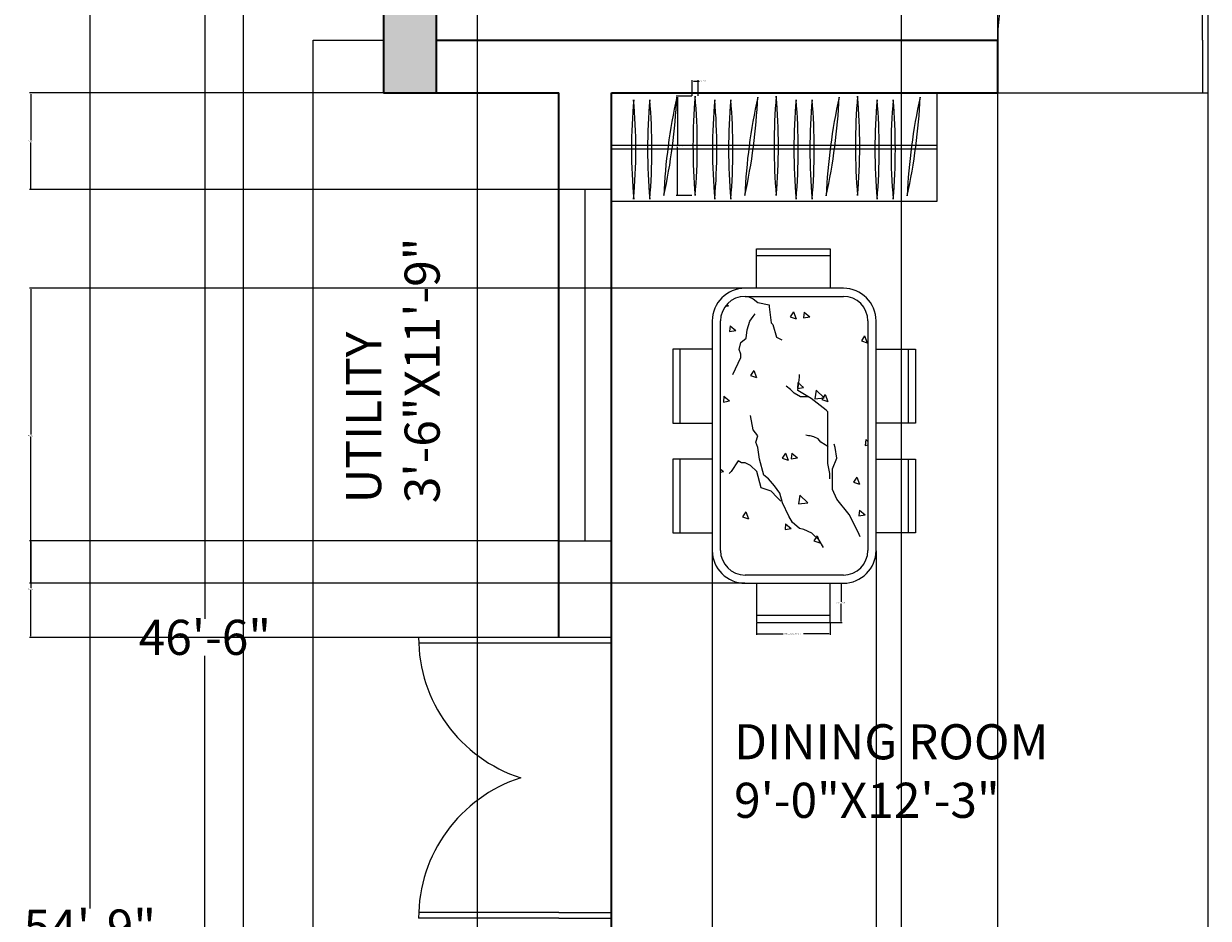
# Model space of a CAD drawing. Units: inches. Extents: x -36 to 401, y -686 to 73.
# Tile 11 of 15: x -36 to 167, y -319 to -166. Entities that reach past the tile are written whole.
import ezdxf

# ---------------------------------------------------------------- set-up
doc = ezdxf.new("R2010")
doc.units = ezdxf.units.IN
doc.header["$MEASUREMENT"] = 0
for name, color, linetype, lineweight in [('A-ANNO-DIMS', 2, 'Continuous', 18), ('A-AREA-IDEN', 7, 'Continuous', 18), ('A-COLS-PATT', 22, 'Continuous', 13), ('A-DOOR', 3, 'Continuous', 18), ('A-FLOR', 7, 'Continuous', 25), ('A-FLOR-CASE', 9, 'Continuous', 18), ('A-FURN', 8, 'Continuous', 13), ('A-GLAZ', 4, 'Continuous', 18), ('A-WALL', 7, 'Continuous', 35), ('C-PROP', 7, 'Continuous', 25)]:
    doc.layers.add(name, color=color, linetype=linetype, lineweight=lineweight)
doc.styles.get("Standard").update_dxf_attribs({"font": 'arial.ttf'})
doc.dimstyles.get("Standard").update_dxf_attribs({"dimtxt": 0.18, "dimasz": 0.18, "dimexe": 0.18, "dimexo": 0.0625, "dimgap": 0.09, "dimtad": 0, "dimtih": 1, "dimtoh": 1, "dimdec": 0, "dimzin": 0, "dimdsep": 46, "dimlunit": 3, "dimtxsty": 'Standard', "dimcen": 0.09, "dimadec": 0, "dimazin": 0, "dimtfac": 1, "dimtdec": 0, "dimtofl": 0, "dimtmove": 0, "dimatfit": 3, "dimfxl": 1, "dimtolj": 1, "dimtzin": 0, "dimarcsym": 0})

# ---------------------------------------------------------------- blocks, each defined once
blk = doc.blocks.new('*D8')
at = {"layer": 'A-ANNO-DIMS', "color": 0, "lineweight": -2, "transparency": 16777216}
for p, q in [((25.63, 7.79), (-24.68, 7.79)), ((-24.5, 7.61), (-24.5, -317.56)), ((-24.5, -649.03), (-24.5, -323.86)), ((1.63, -649.21), (-24.68, -649.21))]:
    blk.add_line(p, q, dxfattribs=at)
at = {"layer": 'A-ANNO-DIMS', "color": 0, "transparency": 16777216}
for points in [[(-24.53, 7.61), (-24.47, 7.61), (-24.5, 7.79)], [(-24.53, -649.03), (-24.47, -649.03), (-24.5, -649.21)]]:
    blk.add_solid(points, dxfattribs=at)
at = {"layer": 'Defpoints', "color": 0, "transparency": 16777216}
for p in [(25.69, 7.79), (-24.5, -649.21), (1.69, -649.21)]:
    blk.add_point(p, dxfattribs=at)
at = {"layer": 'A-ANNO-DIMS', "color": 0, "transparency": 16777216, "insert": (-24.5, -320.71), "char_height": 6, "attachment_point": 5}
blk.add_mtext('\\A1;54\'-9"', dxfattribs=at)
blk = doc.blocks.new('*D11')
at = {"layer": 'A-ANNO-DIMS', "color": 0, "lineweight": -2, "transparency": 16777216}
for p, q in [((25.63, 7.79), (-5.02, 7.79)), ((-4.84, 7.61), (-4.84, -268.06)), ((-4.84, -550.03), (-4.84, -274.36)), ((25.63, -550.21), (-5.02, -550.21))]:
    blk.add_line(p, q, dxfattribs=at)
at = {"layer": 'A-ANNO-DIMS', "color": 0, "transparency": 16777216}
for points in [[(-4.87, 7.61), (-4.81, 7.61), (-4.84, 7.79)], [(-4.87, -550.03), (-4.81, -550.03), (-4.84, -550.21)]]:
    blk.add_solid(points, dxfattribs=at)
at = {"layer": 'Defpoints', "color": 0, "transparency": 16777216}
for p in [(25.69, 7.79), (-4.84, -550.21), (25.69, -550.21)]:
    blk.add_point(p, dxfattribs=at)
at = {"layer": 'A-ANNO-DIMS', "color": 0, "transparency": 16777216, "insert": (-4.84, -271.21), "char_height": 6, "attachment_point": 5}
blk.add_mtext('\\A1;46\'-6"', dxfattribs=at)
blk = doc.blocks.new('WIN-60IN')
for p, q in [((0, 9), (60, 9)), ((0, 0), (0, 9)), ((60, 9), (60, 0)), ((0, 4.5), (60, 4.5)), ((60, 0), (0, 0))]:
    blk.add_line(p, q)
blk = doc.blocks.new('DOOR-SWING-36IN')
for p, q in [((-1, 0), (-1, 36)), ((0, 0), (0, 36))]:
    blk.add_line(p, q)
blk.add_arc((0, 0), 36, 90, 180)
blk = doc.blocks.new('DOOR-PAIR-48IN')
for p, q in [((0, 48), (-24, 48)), ((0, 47), (-24, 47)), ((9, 48), (0, 48)), ((9, 47), (0, 47)), ((0, 1), (-24, 1)), ((0, 0), (-24, 0)), ((0, 1), (9, 1)), ((0, 0), (9, 0))]:
    blk.add_line(p, q)
for centre, start, end in [((1.23, 48), 180, 252.0547), ((1.23, 0), 107.9453, 180)]:
    blk.add_arc(centre, 25.23, start, end)
blk = doc.blocks.new('CHAIR-DINING')
for p, q in [((0, 6.75), (0, 0)), ((12.6, 0), (12.6, 6.75)), ((12.6, 1.23), (0, 1.23)), ((0, 0), (12.6, 0))]:
    blk.add_line(p, q)
blk = doc.blocks.new('GARMENT-ON-RAIL-SMALL')
for centre, start, end in [((97.52, 8.49), 175.0028, 184.9972), ((-96.78, 8.49), 355.0028, 4.9972)]:
    blk.add_arc(centre, 97.52, start, end)
blk = doc.blocks.new('*D33')
at = {"layer": 'A-ANNO-DIMS', "color": 0, "lineweight": -2, "transparency": 16777216}
for p, q in [((78.42, -178.75), (75.75, -178.75)), ((75.93, -178.93), (75.93, -187.07)), ((75.93, -195.56), (75.93, -187.43)), ((78.42, -195.74), (75.75, -195.74))]:
    blk.add_line(p, q, dxfattribs=at)
at = {"layer": 'A-ANNO-DIMS', "color": 0, "transparency": 16777216}
for points in [[(75.9, -178.93), (75.96, -178.93), (75.93, -178.75)], [(75.9, -195.56), (75.96, -195.56), (75.93, -195.74)]]:
    blk.add_solid(points, dxfattribs=at)
at = {"layer": 'Defpoints', "color": 0, "transparency": 16777216}
for p in [(75.93, -178.75), (78.48, -178.75), (78.48, -195.74)]:
    blk.add_point(p, dxfattribs=at)
at = {"layer": 'A-ANNO-DIMS', "color": 0, "transparency": 16777216, "insert": (75.93, -187.25), "char_height": 0.18, "attachment_point": 5}
blk.add_mtext('\\A1;HANGER 1\'-5" TYP.', dxfattribs=at)
blk = doc.blocks.new('*D34')
at = {"layer": 'A-ANNO-DIMS', "color": 0, "lineweight": -2, "transparency": 16777216}
for p, q in [((78.48, -178.69), (78.48, -176.03)), ((79.47, -178.69), (79.47, -176.03)), ((78.66, -176.21), (79.29, -176.21)), ((79.47, -176.21), (79.65, -176.21))]:
    blk.add_line(p, q, dxfattribs=at)
at = {"layer": 'A-ANNO-DIMS', "color": 0, "transparency": 16777216}
for points in [[(78.66, -176.18), (78.66, -176.24), (78.48, -176.21)], [(79.29, -176.18), (79.29, -176.24), (79.47, -176.21)]]:
    blk.add_solid(points, dxfattribs=at)
at = {"layer": 'Defpoints', "color": 0, "transparency": 16777216}
for p in [(79.47, -176.21), (78.48, -178.75), (79.47, -178.75)]:
    blk.add_point(p, dxfattribs=at)
at = {"layer": 'A-ANNO-DIMS', "color": 0, "transparency": 16777216, "insert": (80.29, -176.21), "char_height": 0.18, "attachment_point": 5}
blk.add_mtext('\\A1;0\'-1" TYP.', dxfattribs=at)
blk = doc.blocks.new('*D35')
at = {"layer": 'A-ANNO-DIMS', "color": 0, "lineweight": -2, "transparency": 16777216}
for p, q in [((89.43, -268.77), (89.43, -270.77)), ((102.03, -268.77), (102.03, -270.77)), ((89.61, -270.59), (93.99, -270.59)), ((101.85, -270.59), (97.48, -270.59))]:
    blk.add_line(p, q, dxfattribs=at)
at = {"layer": 'A-ANNO-DIMS', "color": 0, "transparency": 16777216}
for points in [[(89.61, -270.56), (89.61, -270.62), (89.43, -270.59)], [(101.85, -270.56), (101.85, -270.62), (102.03, -270.59)]]:
    blk.add_solid(points, dxfattribs=at)
at = {"layer": 'Defpoints', "color": 0, "transparency": 16777216}
for p in [(89.43, -268.7), (102.03, -268.7), (102.03, -270.59)]:
    blk.add_point(p, dxfattribs=at)
at = {"layer": 'A-ANNO-DIMS', "color": 0, "transparency": 16777216, "insert": (95.73, -270.59), "char_height": 0.18, "attachment_point": 5}
blk.add_mtext('\\A1;DINING CHAIR 1\'-0 1/2" TYP.', dxfattribs=at)
blk = doc.blocks.new('*D36')
at = {"layer": 'A-ANNO-DIMS', "color": 0, "lineweight": -2, "transparency": 16777216}
for p, q in [((102.1, -261.96), (104.1, -261.96)), ((103.92, -262.14), (103.92, -265.15)), ((103.92, -268.52), (103.92, -265.51)), ((102.1, -268.7), (104.1, -268.7))]:
    blk.add_line(p, q, dxfattribs=at)
at = {"layer": 'A-ANNO-DIMS', "color": 0, "transparency": 16777216}
for points in [[(103.89, -262.14), (103.95, -262.14), (103.92, -261.96)], [(103.89, -268.52), (103.95, -268.52), (103.92, -268.7)]]:
    blk.add_solid(points, dxfattribs=at)
at = {"layer": 'Defpoints', "color": 0, "transparency": 16777216}
for p in [(102.03, -261.96), (103.92, -261.96), (102.03, -268.7)]:
    blk.add_point(p, dxfattribs=at)
at = {"layer": 'A-ANNO-DIMS', "color": 0, "transparency": 16777216, "insert": (103.92, -265.33), "char_height": 0.18, "attachment_point": 5}
blk.add_mtext('\\A1;0\'-6 1/2" TYP.', dxfattribs=at)
blk = doc.blocks.new('*D77')
at = {"layer": 'A-ANNO-DIMS', "color": 0, "lineweight": -2, "transparency": 16777216}
for p, q in [((55.63, -178.21), (-34.79, -178.21)), ((-34.61, -178.39), (-34.61, -186.28)), ((-34.61, -194.53), (-34.61, -186.64)), ((55.63, -194.71), (-34.79, -194.71))]:
    blk.add_line(p, q, dxfattribs=at)
at = {"layer": 'A-ANNO-DIMS', "color": 0, "transparency": 16777216}
for points in [[(-34.64, -178.39), (-34.58, -178.39), (-34.61, -178.21)], [(-34.64, -194.53), (-34.58, -194.53), (-34.61, -194.71)]]:
    blk.add_solid(points, dxfattribs=at)
at = {"layer": 'Defpoints', "color": 0, "transparency": 16777216}
for p in [(55.69, -178.21), (-34.61, -194.71), (55.69, -194.71)]:
    blk.add_point(p, dxfattribs=at)
at = {"layer": 'A-ANNO-DIMS', "color": 0, "transparency": 16777216, "insert": (-34.61, -186.46), "char_height": 0.18, "attachment_point": 5}
blk.add_mtext('\\A1;1\'-4 1/2"', dxfattribs=at)
blk = doc.blocks.new('*D78')
at = {"layer": 'A-ANNO-DIMS', "color": 0, "lineweight": -2, "transparency": 16777216}
for p, q in [((55.63, -254.71), (-34.79, -254.71)), ((-34.61, -254.89), (-34.61, -262.78)), ((-34.61, -271.03), (-34.61, -263.14)), ((55.63, -271.21), (-34.79, -271.21))]:
    blk.add_line(p, q, dxfattribs=at)
at = {"layer": 'A-ANNO-DIMS', "color": 0, "transparency": 16777216}
for points in [[(-34.64, -254.89), (-34.58, -254.89), (-34.61, -254.71)], [(-34.64, -271.03), (-34.58, -271.03), (-34.61, -271.21)]]:
    blk.add_solid(points, dxfattribs=at)
at = {"layer": 'Defpoints', "color": 0, "transparency": 16777216}
for p in [(55.69, -254.71), (-34.61, -271.21), (55.69, -271.21)]:
    blk.add_point(p, dxfattribs=at)
at = {"layer": 'A-ANNO-DIMS', "color": 0, "transparency": 16777216, "insert": (-34.61, -262.96), "char_height": 0.18, "attachment_point": 5}
blk.add_mtext('\\A1;1\'-4 1/2"', dxfattribs=at)
blk = doc.blocks.new('*D79')
at = {"layer": 'A-ANNO-DIMS', "color": 0, "lineweight": -2, "transparency": 16777216}
for p, q in [((130.69, -398.65), (130.69, 68.27)), ((130.87, 68.09), (148.36, 68.09)), ((166.51, 68.09), (149.02, 68.09)), ((166.69, -398.65), (166.69, 68.27))]:
    blk.add_line(p, q, dxfattribs=at)
at = {"layer": 'A-ANNO-DIMS', "color": 0, "transparency": 16777216}
for points in [[(130.87, 68.12), (130.87, 68.06), (130.69, 68.09)], [(166.51, 68.12), (166.51, 68.06), (166.69, 68.09)]]:
    blk.add_solid(points, dxfattribs=at)
at = {"layer": 'Defpoints', "color": 0, "transparency": 16777216}
for p in [(166.69, 68.09), (130.69, -398.71), (166.69, -398.71)]:
    blk.add_point(p, dxfattribs=at)
at = {"layer": 'A-ANNO-DIMS', "color": 0, "transparency": 16777216, "insert": (148.69, 68.09), "char_height": 0.18, "attachment_point": 5}
blk.add_mtext('\\A1;3\'-0"', dxfattribs=at)
blk = doc.blocks.new('*D85')
at = {"layer": 'A-ANNO-DIMS', "color": 0, "lineweight": -2, "transparency": 16777216}
for p, q in [((114.18, -126.31), (114.18, -685.69)), ((41.7, -137.56), (41.7, -685.69)), ((41.88, -685.51), (77.4, -685.51)), ((114, -685.51), (78.48, -685.51))]:
    blk.add_line(p, q, dxfattribs=at)
at = {"layer": 'A-ANNO-DIMS', "color": 0, "transparency": 16777216}
for points in [[(41.88, -685.48), (41.88, -685.54), (41.7, -685.51)], [(114, -685.48), (114, -685.54), (114.18, -685.51)]]:
    blk.add_solid(points, dxfattribs=at)
at = {"layer": 'Defpoints', "color": 0, "transparency": 16777216}
for p in [(114.18, -126.25), (41.7, -137.5), (114.18, -685.51)]:
    blk.add_point(p, dxfattribs=at)
at = {"layer": 'A-ANNO-DIMS', "color": 0, "transparency": 16777216, "insert": (77.94, -685.51), "char_height": 0.18, "attachment_point": 5}
blk.add_mtext('\\A1;6\'-0 1/2"', dxfattribs=at)
blk = doc.blocks.new('*D89')
at = {"layer": 'A-ANNO-DIMS', "color": 0, "lineweight": -2, "transparency": 16777216}
for p, q in [((81.9, -256.42), (81.9, -685.69)), ((109.9, -256.42), (109.9, -685.69)), ((82.08, -685.51), (95.57, -685.51)), ((109.72, -685.51), (96.23, -685.51))]:
    blk.add_line(p, q, dxfattribs=at)
at = {"layer": 'A-ANNO-DIMS', "color": 0, "transparency": 16777216}
for points in [[(82.08, -685.48), (82.08, -685.54), (81.9, -685.51)], [(109.72, -685.48), (109.72, -685.54), (109.9, -685.51)]]:
    blk.add_solid(points, dxfattribs=at)
at = {"layer": 'Defpoints', "color": 0, "transparency": 16777216}
for p in [(81.9, -256.36), (109.9, -256.36), (109.9, -685.51)]:
    blk.add_point(p, dxfattribs=at)
at = {"layer": 'A-ANNO-DIMS', "color": 0, "transparency": 16777216, "insert": (95.9, -685.51), "char_height": 0.18, "attachment_point": 5}
blk.add_mtext('\\A1;2\'-4"', dxfattribs=at)
blk = doc.blocks.new('*D90')
at = {"layer": 'A-ANNO-DIMS', "color": 0, "lineweight": -2, "transparency": 16777216}
for p, q in [((87.44, -211.56), (-34.79, -211.56)), ((-34.61, -211.74), (-34.61, -236.57)), ((-34.61, -261.78), (-34.61, -236.94)), ((87.44, -261.96), (-34.79, -261.96))]:
    blk.add_line(p, q, dxfattribs=at)
at = {"layer": 'A-ANNO-DIMS', "color": 0, "transparency": 16777216}
for points in [[(-34.64, -211.74), (-34.58, -211.74), (-34.61, -211.56)], [(-34.64, -261.78), (-34.58, -261.78), (-34.61, -261.96)]]:
    blk.add_solid(points, dxfattribs=at)
at = {"layer": 'Defpoints', "color": 0, "transparency": 16777216}
for p in [(87.5, -211.56), (-34.61, -261.96), (87.5, -261.96)]:
    blk.add_point(p, dxfattribs=at)
at = {"layer": 'A-ANNO-DIMS', "color": 0, "transparency": 16777216, "insert": (-34.61, -236.76), "char_height": 0.18, "attachment_point": 5}
blk.add_mtext('\\A1;4\'-2 1/2"', dxfattribs=at)

msp = doc.modelspace()

# ---------------------------------------------------------------- hatches: boundary and pattern name
at = {"layer": 'A-COLS-PATT'}
h = msp.add_hatch(color=256, dxfattribs=at)
h.dxf.hatch_style = 1
h.paths.add_polyline_path([(34.69, 7.79), (25.69, 7.79), (25.69, -13.21), (34.69, -13.21)])
h.paths.add_polyline_path([(172.69, -13.21), (177.19, -13.21), (181.69, -13.21), (181.69, 7.79), (172.69, 7.79)])
h.paths.add_polyline_path([(322.69, 7.79), (313.69, 7.79), (313.69, -13.21), (322.69, -13.21)])
h.paths.add_polyline_path([(322.69, -157.21), (313.69, -157.21), (313.69, -178.21), (322.69, -178.21)])
h.paths.add_polyline_path([(172.69, -178.21), (177.19, -178.21), (181.69, -178.21), (181.69, -157.21), (177.19, -157.21), (172.69, -157.21)])
h.paths.add_polyline_path([(25.69, -178.21), (34.69, -178.21), (34.69, -157.21), (25.69, -157.21)])
h.paths.add_polyline_path([(34.69, -325.21), (25.69, -325.21), (25.69, -346.21), (34.69, -346.21)])
h.paths.add_polyline_path([(181.69, -325.21), (177.19, -325.21), (172.69, -325.21), (172.69, -346.21), (177.19, -346.21), (181.69, -346.21)])
h.paths.add_polyline_path([(322.69, -325.21), (313.69, -325.21), (313.69, -346.21), (322.69, -346.21)])
h.paths.add_polyline_path([(364.69, -451.21), (358.69, -451.21), (358.69, -472.21), (364.69, -472.21)])
h.paths.add_polyline_path([(181.69, -451.21), (177.19, -451.21), (172.69, -451.21), (172.69, -472.21), (177.19, -472.21), (181.69, -472.21)])
h.paths.add_polyline_path([(25.69, -472.21), (34.69, -472.21), (34.69, -451.21), (25.69, -451.21)])

# ---------------------------------------------------------------- linework, layer by layer
at = {"layer": 'A-DOOR'}
for p, q in [((165.69, -169.21), (165.69, -178.21)), ((130.69, -178.21), (166.69, -178.21))]:
    msp.add_line(p, q, dxfattribs=at)
at = {"layer": 'A-FLOR'}
for p, q in [((13.69, -178.21), (13.69, -169.21)), ((13.69, -169.21), (25.69, -169.21)), ((25.69, -178.21), (13.69, -178.21)), ((13.69, -325.21), (13.69, -178.21))]:
    msp.add_line(p, q, dxfattribs=at)
at = {"layer": 'A-FLOR-CASE'}
for p, q in [((120.29, -178.21), (64.69, -178.21)), ((64.69, -178.21), (64.69, -196.74)), ((120.29, -178.21), (120.29, -196.74)), ((120.29, -187.17), (64.69, -187.17)), ((120.29, -187.79), (64.69, -187.79)), ((120.29, -196.74), (64.69, -196.74))]:
    msp.add_line(p, q, dxfattribs=at)
at = {"layer": 'A-FURN'}
for p, q in [((104.3, -211.56), (87.5, -211.56)), ((84.14, -214.64), (84.65, -214.58)), ((84.39, -214.33), (84.65, -214.58)), ((87.5, -212.96), (104.3, -212.96)), ((88.14, -213.06), (88.9, -213.37)), ((88.9, -213.37), (89.66, -213.98)), ((89.66, -213.98), (91.64, -214.43)), ((91.64, -214.43), (91.64, -214.74)), ((88.3, -217.18), (88.91, -216.41)), ((88.91, -216.41), (89.21, -215.96)), ((91.64, -214.74), (91.94, -217.48)), ((95.76, -215.61), (95.2, -216.45)), ((95.2, -216.45), (96.21, -216.79)), ((95.76, -215.61), (96.21, -216.79)), ((97.59, -215.64), (97.5, -216.64)), ((97.5, -216.65), (98.55, -216.45)), ((97.59, -215.64), (98.55, -216.45)), ((81.9, -217.16), (81.9, -256.36)), ((83.3, -256.36), (83.3, -217.16)), ((84.95, -217.97), (84.86, -218.98)), ((84.95, -217.97), (85.92, -218.78)), ((87.84, -218.7), (88.3, -217.18)), ((91.94, -217.48), (92.25, -217.78)), ((92.25, -217.78), (92.85, -219.91)), ((108.5, -217.16), (108.5, -256.36)), ((109.9, -256.36), (109.9, -217.16)), ((84.86, -218.98), (85.92, -218.78)), ((86.78, -220.83), (87.69, -220.07)), ((87.69, -220.07), (87.84, -218.7)), ((92.85, -219.91), (93.77, -220.37)), ((107.94, -219.7), (107.38, -220.54)), ((107.38, -220.54), (108.39, -220.88)), ((107.94, -219.7), (108.39, -220.88)), ((86.47, -222.05), (86.78, -220.83)), ((86.78, -222.81), (86.47, -222.05)), ((85.41, -226.31), (86.78, -223.42)), ((86.78, -223.42), (86.78, -222.81)), ((89, -225.64), (88.43, -226.48)), ((88.43, -226.48), (89.45, -226.82)), ((89, -225.64), (89.45, -226.82)), ((96.5, -229.05), (96.81, -226.76)), ((96.81, -226.76), (96.81, -226.31)), ((95.29, -228.89), (94.53, -228.29)), ((96.53, -227.69), (96.45, -228.69)), ((96.45, -228.69), (97.5, -228.5)), ((96.53, -227.69), (97.5, -228.5)), ((83.9, -230.02), (83.81, -231.03)), ((83.81, -231.03), (84.86, -230.83)), ((83.9, -230.02), (84.86, -230.83)), ((95.89, -229.5), (95.29, -228.89)), ((96.96, -230.11), (95.89, -229.5)), ((98.78, -230.42), (96.5, -229.05)), ((98.33, -230.11), (96.96, -230.11)), ((101.37, -232.4), (98.78, -230.42)), ((99.65, -228.97), (99.42, -230.47)), ((99.42, -230.47), (101.01, -230.28)), ((99.65, -228.97), (101.01, -230.28)), ((101.18, -229.73), (100.61, -230.56)), ((100.61, -230.56), (101.63, -230.9)), ((101.18, -229.73), (101.63, -230.9)), ((101.67, -232.7), (101.37, -232.4)), ((101.67, -241.53), (101.67, -232.7)), ((88.9, -235.74), (88.44, -233.31)), ((89.66, -236.81), (88.9, -235.74)), ((89.36, -237.88), (89.66, -236.81)), ((98.33, -236.81), (97.88, -236.66)), ((98.64, -236.81), (98.33, -236.81)), ((99.25, -236.96), (98.64, -236.81)), ((89.66, -238.79), (89.36, -237.88)), ((89.96, -240.77), (89.66, -238.79)), ((100.01, -237.27), (99.25, -236.96)), ((100.46, -237.88), (100.01, -237.27)), ((101.22, -238.33), (100.46, -237.88)), ((101.68, -238.64), (101.22, -238.33)), ((102.89, -238.79), (102.74, -238.18)), ((103.19, -240.62), (102.89, -238.79)), ((108.12, -237.41), (108.03, -238.41)), ((108.03, -238.41), (108.5, -238.33)), ((108.12, -237.41), (108.5, -237.73)), ((90.73, -243.51), (89.96, -240.77)), ((94.41, -239.76), (93.85, -240.59)), ((93.85, -240.59), (94.87, -240.93)), ((94.41, -239.76), (94.87, -240.93)), ((95.48, -239.74), (95.39, -240.74)), ((95.39, -240.74), (96.44, -240.55)), ((95.48, -239.74), (96.44, -240.55)), ((102.43, -242.44), (103.19, -240.62)), ((83.3, -242.46), (83.81, -242.88)), ((83.3, -242.97), (83.81, -242.88)), ((85.1, -242.9), (84.8, -243.2)), ((86.32, -241.07), (85.1, -242.9)), ((86.92, -241.38), (86.32, -241.07)), ((87.53, -241.38), (86.92, -241.38)), ((88.44, -241.83), (87.53, -241.38)), ((89.51, -242.9), (88.44, -241.83)), ((90.27, -245.64), (89.51, -242.9)), ((101.98, -243.2), (101.67, -241.53)), ((102.43, -245.94), (102.43, -242.44)), ((91.49, -244.12), (90.73, -243.51)), ((92.55, -245.34), (91.49, -244.12)), ((101.98, -244.12), (101.98, -243.2)), ((106.6, -243.84), (106.03, -244.68)), ((106.03, -244.68), (107.05, -245.02)), ((106.6, -243.84), (107.05, -245.02)), ((90.57, -245.79), (90.27, -245.64)), ((91.94, -246.25), (90.57, -245.79)), ((93.01, -247.31), (91.94, -246.25)), ((93.46, -246.55), (92.55, -245.34)), ((93.92, -248.23), (93.46, -246.55)), ((96.87, -246.9), (96.64, -248.4)), ((96.87, -246.9), (98.23, -248.21)), ((103.19, -247.62), (102.43, -245.94)), ((93.61, -247.92), (93.01, -247.31)), ((94.98, -250.51), (93.92, -248.23)), ((96.64, -248.4), (98.23, -248.21)), ((105.32, -250.21), (103.19, -247.62)), ((87.65, -249.78), (87.09, -250.62)), ((87.09, -250.62), (88.1, -250.96)), ((87.65, -249.78), (88.1, -250.96)), ((95.59, -251.58), (94.98, -250.51)), ((106.84, -253.25), (105.32, -250.21)), ((107.06, -249.46), (106.97, -250.46)), ((106.97, -250.46), (108.03, -250.27)), ((107.06, -249.46), (108.03, -250.27)), ((94.43, -251.79), (94.34, -252.79)), ((94.34, -252.79), (95.39, -252.6)), ((94.43, -251.79), (95.39, -252.6)), ((96.35, -252.19), (95.59, -251.58)), ((96.81, -252.64), (96.35, -252.19)), ((97.57, -252.79), (96.81, -252.64)), ((98.94, -253.4), (97.57, -252.79)), ((100.15, -254.62), (98.94, -253.4)), ((99.83, -253.87), (99.27, -254.71)), ((99.27, -254.71), (100.28, -255.05)), ((99.83, -253.87), (100.28, -255.05)), ((100.91, -255.84), (100.15, -254.62)), ((107.15, -254.01), (106.84, -253.25)), ((104.3, -260.56), (87.5, -260.56)), ((87.5, -261.96), (104.3, -261.96))]:
    msp.add_line(p, q, dxfattribs=at)
for centre, radius, start, end in [((87.5, -217.16), 5.6, 90, 180), ((104.3, -217.16), 5.6, 0, 90), ((87.5, -217.16), 4.2, 90, 180), ((104.3, -217.16), 4.2, 0, 90), ((87.5, -256.36), 5.6, 180, 270), ((87.5, -256.36), 4.2, 180, 270), ((104.3, -256.36), 4.2, 270, 0), ((104.3, -256.36), 5.6, 270, 0)]:
    msp.add_arc(centre, radius, start, end, dxfattribs=at)
at = {"layer": 'A-WALL'}
for p, q in [((25.69, 7.79), (25.69, -178.21)), ((34.69, 7.79), (34.69, -178.21)), ((34.69, -169.21), (130.69, -169.21)), ((130.69, -178.21), (130.69, -169.21)), ((25.69, -178.21), (55.69, -178.21)), ((55.69, -271.21), (55.69, -178.21)), ((64.69, -334.21), (64.69, -178.21)), ((64.69, -178.21), (130.69, -178.21))]:
    msp.add_line(p, q, dxfattribs=at)
at = {"layer": 'C-PROP'}
msp.add_line((1.69, 31.79), (1.69, -649.21), dxfattribs=at)

# ---------------------------------------------------------------- block references
at = {"layer": 'A-DOOR'}
for name, p in [('DOOR-SWING-36IN', (166.69, -169.21)), ('DOOR-PAIR-48IN', (55.69, -319.21))]:
    msp.add_blockref(name, p, dxfattribs=at)
at = {"layer": 'A-FLOR-CASE'}
for p in [(68.09, -196.34), (70.84, -196.34), (78.6, -195.74), (81.94, -196.34), (84.69, -196.34), (92.46, -195.74), (95.85, -196.34), (98.59, -196.34), (106.36, -195.74), (109.7, -196.34), (112.45, -196.34)]:
    msp.add_blockref('GARMENT-ON-RAIL-SMALL', p, dxfattribs=at)
for p, rotation in [((76.19, -178.95), 172.5051423894903), ((90.04, -178.95), 172.5051423894903), ((101, -195.7), 352.5051423895286), ((114.85, -195.7), 352.5051423896668)]:
    msp.add_blockref('GARMENT-ON-RAIL-SMALL', p, dxfattribs=dict(at, rotation=rotation))
at = {"layer": 'A-FURN', "extrusion": (0, 0, -1), "zscale": -1}
for p, rotation in [((-89.43, -204.81), 180), ((-116.65, -222), 270), ((-116.65, -240.76), 270)]:
    msp.add_blockref('CHAIR-DINING', p, dxfattribs=dict(at, rotation=rotation))
at = {"layer": 'A-FURN', "rotation": 270}
for p in [(75.15, -222), (75.15, -240.76)]:
    msp.add_blockref('CHAIR-DINING', p, dxfattribs=at)
at = {"layer": 'A-FURN'}
msp.add_blockref('CHAIR-DINING', (89.43, -268.7), dxfattribs=at)
at = {"layer": 'A-GLAZ', "extrusion": (0, 0, -1), "zscale": -1, "rotation": 90}
msp.add_blockref('WIN-60IN', (-55.69, -254.71), dxfattribs=at)

# ---------------------------------------------------------------- texts
at = {"layer": 'A-AREA-IDEN', "insert": (19.3, -248.3), "char_height": 6, "attachment_point": 1, "rotation": 90}
msp.add_mtext('UTILITY\\P3\'-6"X11\'-9"', dxfattribs=at)
at = {"layer": 'A-AREA-IDEN', "insert": (85.62, -286.05), "char_height": 6, "attachment_point": 1}
msp.add_mtext('DINING ROOM\\P9\'-0"X12\'-3"', dxfattribs=at)

# ---------------------------------------------------------------- dimensions: what is measured, and where the dimension line sits
at = {"layer": 'A-ANNO-DIMS'}
for base, p1, p2, picture, middle in [((166.69, 68.09), (130.69, -398.71), (166.69, -398.71), '*D79', (148.69, 68.09)), ((114.18, -685.51), (41.7, -137.5), (114.18, -126.25), '*D85', (77.94, -685.51)), ((109.9, -685.51), (81.9, -256.36), (109.9, -256.36), '*D89', (95.9, -685.51))]:
    dim = msp.add_linear_dim(base=base, p1=p1, p2=p2, dimstyle='Standard', override={"dimdec": 1, "dimlfac": 1, "dimrnd": 0, "dimzin": 1, "dimdsep": 46, "dimlunit": 4, "dimfrac": 2}, dxfattribs=at)
    dim.commit()
    dim.dimension.update_dxf_attribs({"geometry": picture, "text_midpoint": middle})
for base, p1, p2, override, picture, middle in [((-24.5, -649.21), (25.69, 7.79), (1.69, -649.21), {"dimtxt": 6, "dimclrd": 0, "dimclre": 0, "dimclrt": 0}, '*D8', (-24.5, -320.71)), ((-4.84, -550.21), (25.69, 7.79), (25.69, -550.21), {"dimtxt": 6, "dimclrd": 0, "dimclre": 0, "dimclrt": 0}, '*D11', (-4.84, -271.21)), ((-34.61, -194.71), (55.69, -178.21), (55.69, -194.71), {"dimdec": 1, "dimlfac": 1, "dimrnd": 0, "dimzin": 1, "dimdsep": 46, "dimlunit": 4, "dimfrac": 2}, '*D77', (-34.61, -186.46)), ((-34.61, -261.96), (87.5, -211.56), (87.5, -261.96), {"dimdec": 1, "dimlfac": 1, "dimrnd": 0, "dimzin": 1, "dimdsep": 46, "dimlunit": 4, "dimfrac": 2}, '*D90', (-34.61, -236.76)), ((-34.61, -271.21), (55.69, -254.71), (55.69, -271.21), {"dimdec": 1, "dimlfac": 1, "dimrnd": 0, "dimzin": 1, "dimdsep": 46, "dimlunit": 4, "dimfrac": 2}, '*D78', (-34.61, -262.96))]:
    dim = msp.add_linear_dim(base=base, p1=p1, p2=p2, angle=90, dimstyle='Standard', override=override, dxfattribs=at)
    dim.commit()
    dim.dimension.update_dxf_attribs({"geometry": picture, "text_midpoint": middle})
for base, p1, p2, text, picture, middle in [((79.47, -176.21), (78.48, -178.75), (79.47, -178.75), '<> TYP.', '*D34', (80.29, -176.21)), ((102.03, -270.59), (89.43, -268.7), (102.03, -268.7), 'DINING CHAIR <> TYP.', '*D35', (95.73, -270.59))]:
    dim = msp.add_linear_dim(base=base, p1=p1, p2=p2, text=text, dimstyle='Standard', override={"dimdec": 1, "dimlfac": 1, "dimrnd": 0, "dimzin": 1, "dimdsep": 46, "dimlunit": 4, "dimfrac": 2}, dxfattribs=at)
    dim.commit()
    dim.dimension.update_dxf_attribs({"geometry": picture, "text_midpoint": middle})
for base, p1, p2, text, picture, middle in [((75.93, -178.75), (78.48, -195.74), (78.48, -178.75), 'HANGER <> TYP.', '*D33', (75.93, -187.25)), ((103.92, -261.96), (102.03, -268.7), (102.03, -261.96), '<> TYP.', '*D36', (103.92, -265.33))]:
    dim = msp.add_linear_dim(base=base, p1=p1, p2=p2, angle=90, text=text, dimstyle='Standard', override={"dimdec": 1, "dimlfac": 1, "dimrnd": 0, "dimzin": 1, "dimdsep": 46, "dimlunit": 4, "dimfrac": 2}, dxfattribs=at)
    dim.commit()
    dim.dimension.update_dxf_attribs({"geometry": picture, "text_midpoint": middle})

doc.saveas('drawing.dxf')
